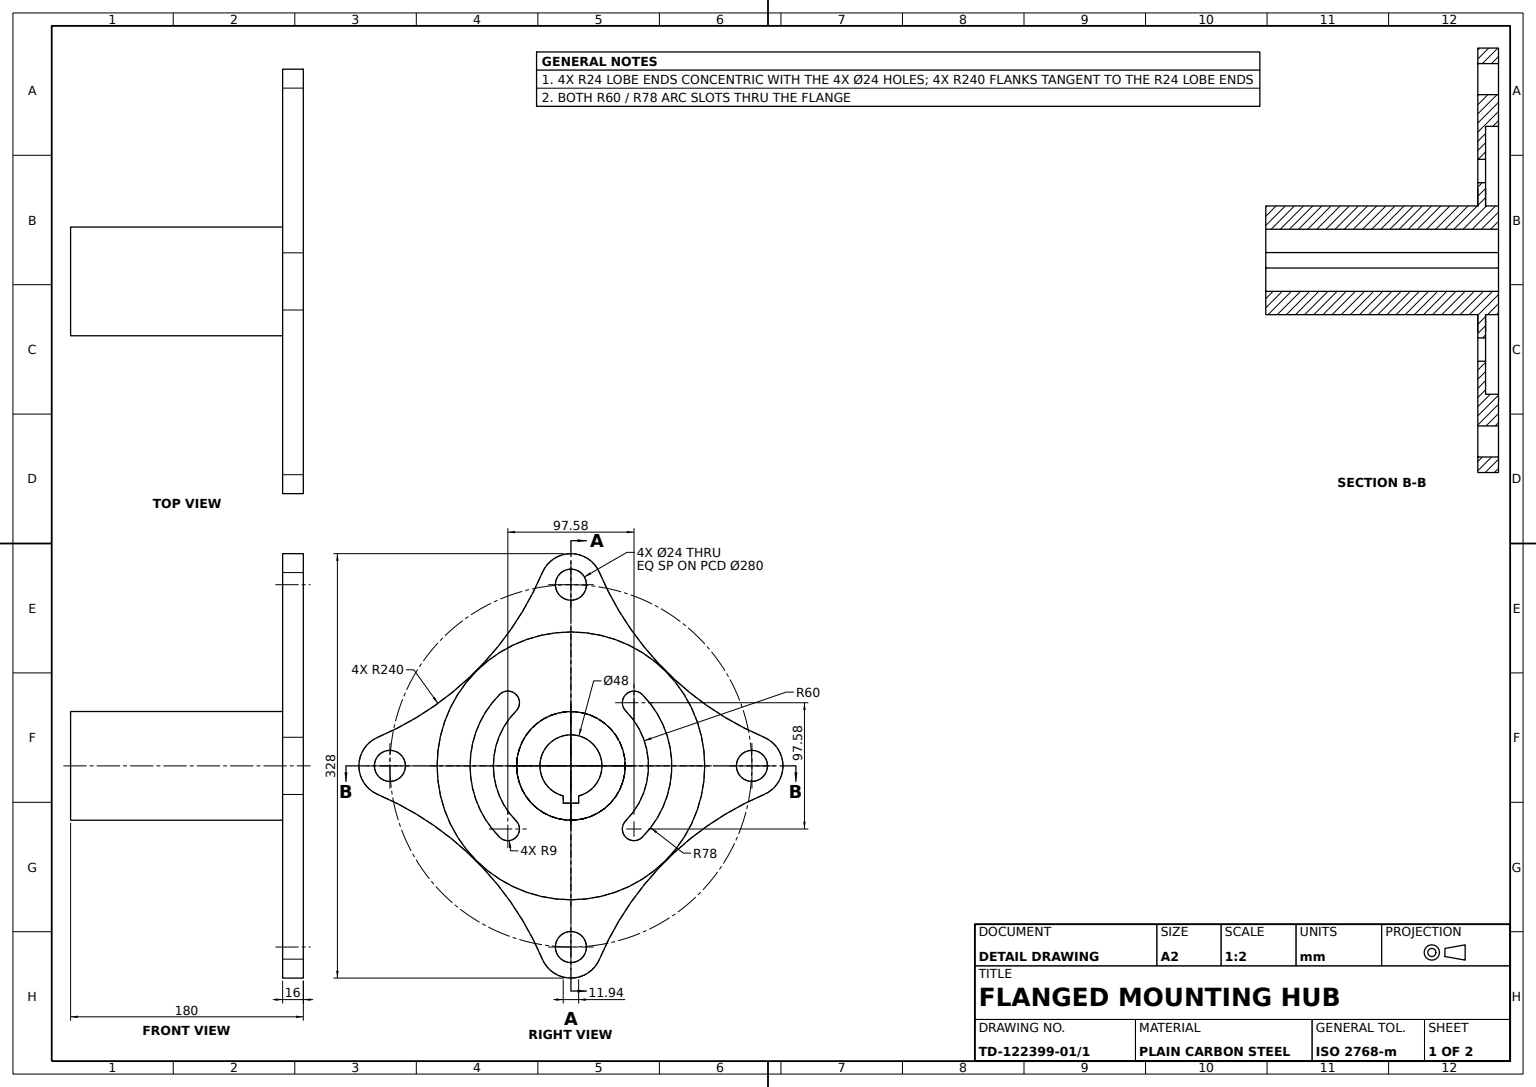
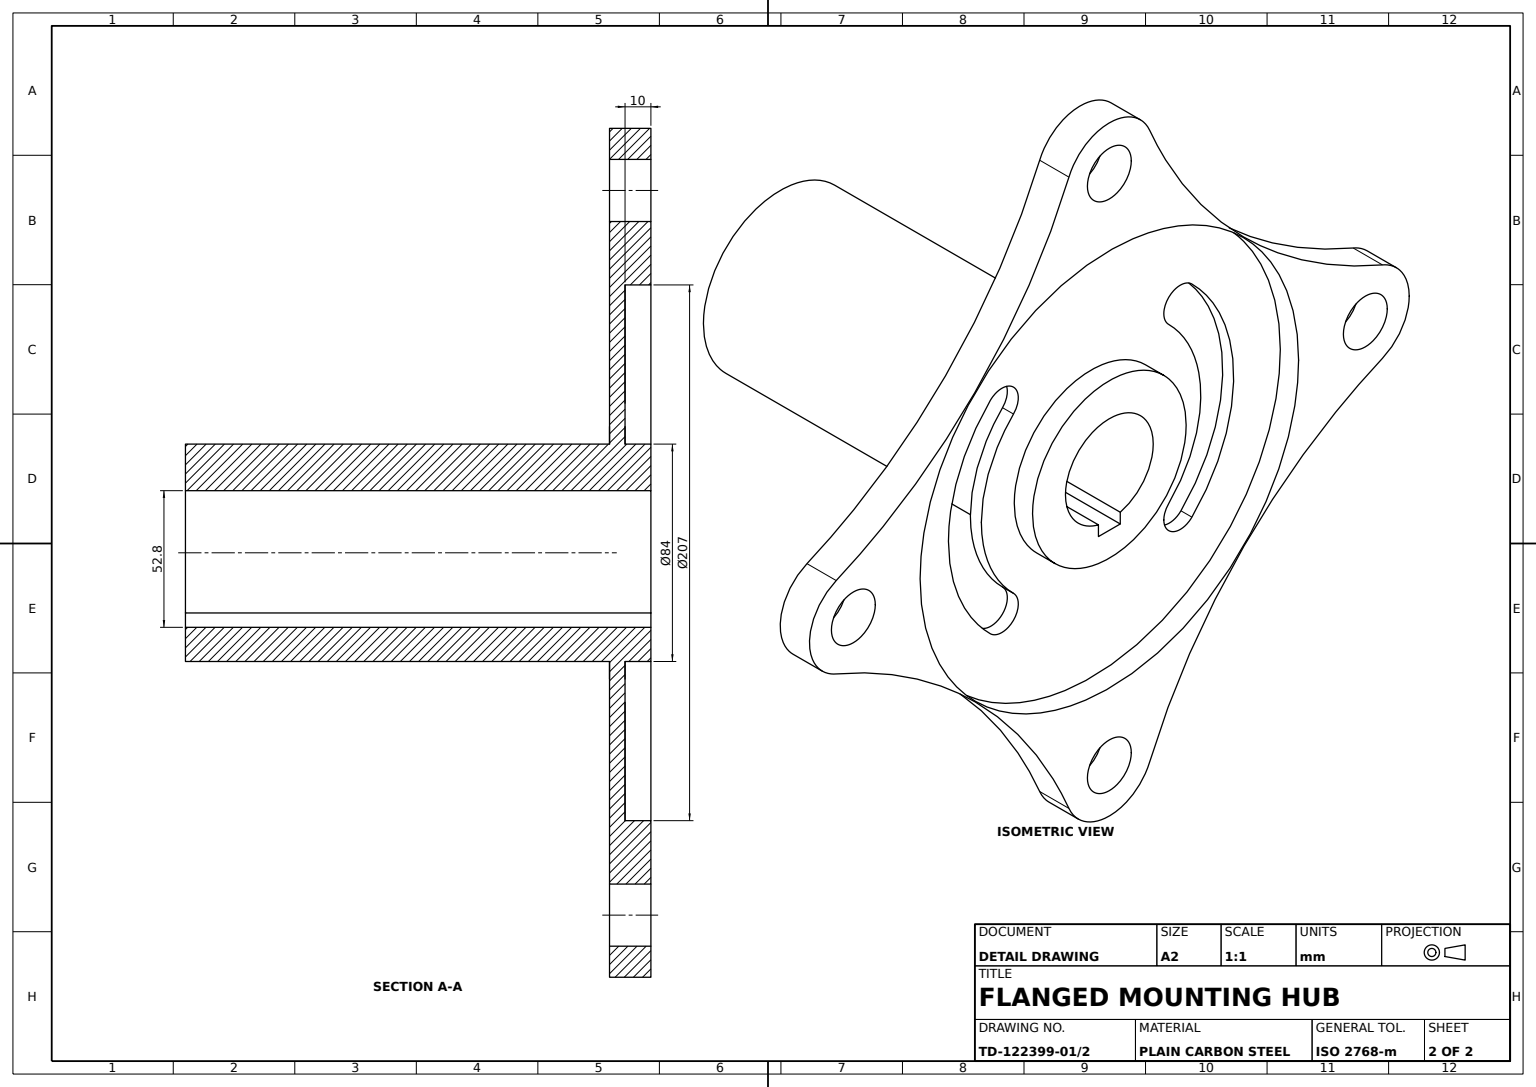
from build123d import *

# Parameters (mm, degrees)
SQUARE_FLANGE_PROFILE_SKETCH_R = 12
SQUARE_FLANGE_240X16_DEPTH     = 16
FLANGE_STEP_CIRCLE_SKETCH_R    = 103.5
FLANGE_STEP_CUT_207_DEPTH      = 10
ARC_SLOTS_R78_DEPTH            = 60
HUB_SKETCH_R                   = 42
HUB_84_DEPTH                   = 180
BORE_SKETCH_R                  = 24
BORE_48_DEPTH                  = 180
KEYWAY_SKETCH_W                = 5.55
KEYWAY_SKETCH_H                = 11.94
KEYWAY_DEPTH                   = 180


with BuildPart() as part:
    # Square Flange Profile Sketch → Square Flange 240x16 (new body)
    with BuildSketch(Plane(origin=(0, 0, 0), x_dir=(1, 0, 0), z_dir=(0, 1, 0))):
        with BuildLine():
            ThreePointArc((22.095900417, 149.368627689), (0, 164), (-22.095900417, 149.368627689))
            ThreePointArc((-22.095900417, 149.368627689), (-73.349277098, 73.349277098), (-149.368627689, 22.095900417))
            ThreePointArc((-149.368627689, 22.095900417), (-164, 0), (-149.368627689, -22.095900417))
            ThreePointArc((-149.368627689, -22.095900417), (-73.349277098, -73.349277098), (-22.095900417, -149.368627689))
            ThreePointArc((-22.095900417, -149.368627689), (0, -164), (22.095900417, -149.368627689))
            ThreePointArc((22.095900417, -149.368627689), (73.349277098, -73.349277098), (149.368627689, -22.095900417))
            ThreePointArc((149.368627689, -22.095900417), (164, 0), (149.368627689, 22.095900417))
            ThreePointArc((149.368627689, 22.095900417), (73.349277098, 73.349277098), (22.095900417, 149.368627689))
        make_face()
        with Locations(Location((0, 140, 0), (0, 0, 270))):
            Circle(SQUARE_FLANGE_PROFILE_SKETCH_R, mode=Mode.SUBTRACT)
        with Locations(Location((140, 0, 0), (0, 0, 270))):
            Circle(SQUARE_FLANGE_PROFILE_SKETCH_R, mode=Mode.SUBTRACT)
        with Locations(Location((0, -140, 0), (0, 0, 270))):
            Circle(SQUARE_FLANGE_PROFILE_SKETCH_R, mode=Mode.SUBTRACT)
        with Locations(Location((-140, 0, 0), (0, 0, 270))):
            Circle(SQUARE_FLANGE_PROFILE_SKETCH_R, mode=Mode.SUBTRACT)
    extrude(amount=SQUARE_FLANGE_240X16_DEPTH)

    # Flange Step Circle Sketch → Flange Step Cut Ø207 (cut)
    with BuildSketch(Plane(origin=(0, 16, 0), x_dir=(1, 0, 0), z_dir=(0, 1, 0))):
        with Locations(Location((0, 0, 0), (0, 0, 270))):
            Circle(FLANGE_STEP_CIRCLE_SKETCH_R)
    extrude(amount=-FLANGE_STEP_CUT_207_DEPTH, mode=Mode.SUBTRACT)

    # Arc Slots Sketch → Arc Slots R78 (cut)
    with BuildSketch(Plane(origin=(0, 6, 0), x_dir=(1, 0, 0), z_dir=(0, 1, 0))):
        with BuildLine():
            ThreePointArc((55.154328933, 55.154328933), (0, 78), (-55.154328933, 55.154328933))
            ThreePointArc((-55.154328933, 55.154328933), (-55.154328933, 42.426406871), (-42.426406871, 42.426406871))
            ThreePointArc((-42.426406871, 42.426406871), (0, 60), (42.426406871, 42.426406871))
            ThreePointArc((42.426406871, 42.426406871), (55.154328933, 42.426406871), (55.154328933, 55.154328933))
        make_face()
        with BuildLine():
            ThreePointArc((42.426406871, -42.426406871), (0, -60), (-42.426406871, -42.426406871))
            ThreePointArc((-42.426406871, -42.426406871), (-55.154328933, -42.426406871), (-55.154328933, -55.154328933))
            ThreePointArc((-55.154328933, -55.154328933), (0, -78), (55.154328933, -55.154328933))
            ThreePointArc((55.154328933, -55.154328933), (55.154328933, -42.426406871), (42.426406871, -42.426406871))
        make_face()
    extrude(amount=-ARC_SLOTS_R78_DEPTH, mode=Mode.SUBTRACT)

    # Hub Sketch → Hub Ø84 (add)
    with BuildSketch(Plane(origin=(0, 16, 0), x_dir=(1, 0, 0), z_dir=(0, 1, 0))):
        with Locations(Location((0, 0, 0), (0, 0, 270))):
            Circle(HUB_SKETCH_R)
    extrude(amount=-HUB_84_DEPTH)

    # Bore Sketch → Bore Ø48 (cut)
    with BuildSketch(Plane(origin=(0, 16, 0), x_dir=(1, 0, 0), z_dir=(0, 1, 0))):
        with Locations(Location((0, 0, 0), (0, 0, 270))):
            Circle(BORE_SKETCH_R)
    extrude(amount=-BORE_48_DEPTH, mode=Mode.SUBTRACT)

    # Keyway Sketch → Keyway (cut)
    with BuildSketch(Plane(origin=(0, 16, 0), x_dir=(1, 0, 0), z_dir=(0, 1, 0))):
        with Locations((26.020625395, 0)):
            Rectangle(KEYWAY_SKETCH_W, KEYWAY_SKETCH_H)
    extrude(amount=-KEYWAY_DEPTH, mode=Mode.SUBTRACT)


solid = part.part
